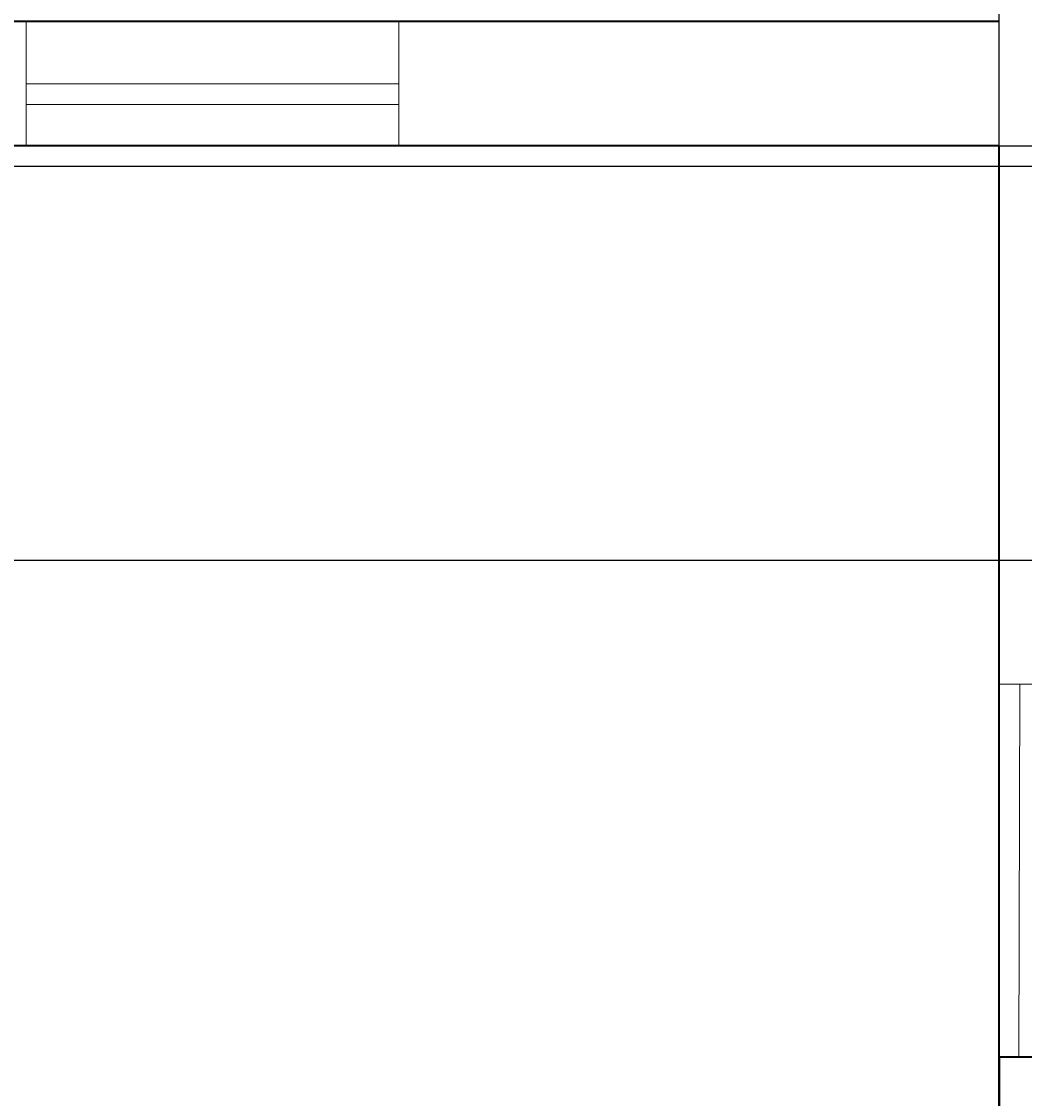
# Model space of a CAD drawing. Units: feet. Extents: x 105 to 1094, y -88 to 588.
# Tile 17 of 59: x 323 to 372, y 250 to 302. Entities that reach past the tile are written whole.
import ezdxf

# ---------------------------------------------------------------- set-up
doc = ezdxf.new("R2010")
doc.units = ezdxf.units.FT
doc.header["$MEASUREMENT"] = 0
for name, color, linetype, lineweight in [('A-ANNO-DIMS', 2, 'Continuous', 18), ('A-GLAZ', 4, 'Continuous', 18), ('A-WALL', 7, 'Continuous', 35)]:
    doc.layers.add(name, color=color, linetype=linetype, lineweight=lineweight)
doc.styles.get("Standard").update_dxf_attribs({"font": 'arial.ttf'})
doc.dimstyles.get("Standard").update_dxf_attribs({"dimtxt": 0.18, "dimasz": 0.18, "dimexe": 0.18, "dimexo": 0.0625, "dimgap": 0.09, "dimtad": 0, "dimtih": 1, "dimtoh": 1, "dimdec": 4, "dimzin": 0, "dimdsep": 46, "dimtxsty": 'Standard', "dimcen": 0.09, "dimadec": 0, "dimazin": 0, "dimtfac": 1, "dimtdec": 4, "dimtofl": 0, "dimtmove": 0, "dimatfit": 3, "dimfxl": 1, "dimtolj": 1, "dimtzin": 0, "dimarcsym": 0})

# ---------------------------------------------------------------- blocks, each defined once
blk = doc.blocks.new('VENT-TRANSVERSE')
for p, q in [((0, 0), (0, 6)), ((18, 0), (18, 6)), ((0, 3), (18, 3)), ((0, 2), (18, 2))]:
    blk.add_line(p, q)
blk = doc.blocks.new('VENT-LONGITUDINAL')
for p, q in [((0, 18), (4, 18)), ((2.039, 0), (2, 18)), ((3.039, 0.002), (3, 18.002))]:
    blk.add_line(p, q)
blk = doc.blocks.new('*D20')
at = {"layer": 'A-ANNO-DIMS', "color": 0, "lineweight": -2, "transparency": 16777216}
for p, q in [((150.688, 276.019), (150.688, -88.149)), ((1048.688, 276.019), (1048.688, -88.149)), ((150.868, -87.969), (599.399, -87.969)), ((1048.508, -87.969), (599.977, -87.969))]:
    blk.add_line(p, q, dxfattribs=at)
at = {"layer": 'A-ANNO-DIMS', "color": 0, "transparency": 16777216}
for points in [[(150.868, -87.939), (150.868, -87.999), (150.688, -87.969)], [(1048.508, -87.939), (1048.508, -87.999), (1048.688, -87.969)]]:
    blk.add_solid(points, dxfattribs=at)
at = {"layer": 'Defpoints', "color": 0, "transparency": 16777216}
for p in [(150.688, 276.081), (1048.688, 276.081), (1048.688, -87.969)]:
    blk.add_point(p, dxfattribs=at)
at = {"layer": 'A-ANNO-DIMS', "color": 0, "transparency": 16777216, "insert": (599.688, -87.969), "char_height": 0.18, "attachment_point": 5}
blk.add_mtext('\\A1;898', dxfattribs=at)
blk = doc.blocks.new('*D21')
at = {"layer": 'A-ANNO-DIMS', "color": 0, "lineweight": -2, "transparency": 16777216}
for p, q in [((849.626, 543.081), (105.458, 543.081)), ((105.638, 542.901), (105.638, 250.263)), ((105.638, -42.739), (105.638, 249.899)), ((849.626, -42.919), (105.458, -42.919))]:
    blk.add_line(p, q, dxfattribs=at)
at = {"layer": 'A-ANNO-DIMS', "color": 0, "transparency": 16777216}
for points in [[(105.608, 542.901), (105.668, 542.901), (105.638, 543.081)], [(105.608, -42.739), (105.668, -42.739), (105.638, -42.919)]]:
    blk.add_solid(points, dxfattribs=at)
at = {"layer": 'Defpoints', "color": 0, "transparency": 16777216}
for p in [(105.638, 543.081), (849.688, 543.081), (849.688, -42.919)]:
    blk.add_point(p, dxfattribs=at)
at = {"layer": 'A-ANNO-DIMS', "color": 0, "transparency": 16777216, "insert": (105.638, 250.081), "char_height": 0.18, "attachment_point": 5}
blk.add_mtext('\\A1;586', dxfattribs=at)
blk = doc.blocks.new('*D33')
at = {"layer": 'A-ANNO-DIMS', "color": 0, "lineweight": -2, "transparency": 16777216}
for p, q in [((646.626, 395.081), (105.458, 395.081)), ((105.638, 394.901), (105.638, 345.263)), ((105.638, 295.261), (105.638, 344.899)), ((646.626, 295.081), (105.458, 295.081))]:
    blk.add_line(p, q, dxfattribs=at)
at = {"layer": 'A-ANNO-DIMS', "color": 0, "transparency": 16777216}
for points in [[(105.608, 394.901), (105.668, 394.901), (105.638, 395.081)], [(105.608, 295.261), (105.668, 295.261), (105.638, 295.081)]]:
    blk.add_solid(points, dxfattribs=at)
at = {"layer": 'Defpoints', "color": 0, "transparency": 16777216}
for p in [(646.688, 395.081), (105.638, 295.081), (646.688, 295.081)]:
    blk.add_point(p, dxfattribs=at)
at = {"layer": 'A-ANNO-DIMS', "color": 0, "transparency": 16777216, "insert": (105.638, 345.081), "char_height": 0.18, "attachment_point": 5}
blk.add_mtext('\\A1;100', dxfattribs=at)
blk = doc.blocks.new('*D39')
at = {"layer": 'A-ANNO-DIMS', "color": 0, "lineweight": -2, "transparency": 16777216}
for p, q in [((294.688, 204.144), (294.688, 588.311)), ((294.868, 588.131), (332.47, 588.131)), ((370.508, 588.131), (332.906, 588.131)), ((370.688, 204.144), (370.688, 588.311))]:
    blk.add_line(p, q, dxfattribs=at)
at = {"layer": 'A-ANNO-DIMS', "color": 0, "transparency": 16777216}
for points in [[(294.868, 588.161), (294.868, 588.101), (294.688, 588.131)], [(370.508, 588.161), (370.508, 588.101), (370.688, 588.131)]]:
    blk.add_solid(points, dxfattribs=at)
at = {"layer": 'Defpoints', "color": 0, "transparency": 16777216}
for p in [(370.688, 588.131), (294.688, 204.081), (370.688, 204.081)]:
    blk.add_point(p, dxfattribs=at)
at = {"layer": 'A-ANNO-DIMS', "color": 0, "transparency": 16777216, "insert": (332.688, 588.131), "char_height": 0.18, "attachment_point": 5}
blk.add_mtext('\\A1;76', dxfattribs=at)
blk = doc.blocks.new('*D54')
at = {"layer": 'A-ANNO-DIMS', "color": 0, "lineweight": -2, "transparency": 16777216}
for p, q in [((294.751, 296.081), (1093.918, 296.081)), ((1093.738, 295.901), (1093.738, 286.263)), ((1093.738, 276.261), (1093.738, 285.899)), ((294.751, 276.081), (1093.918, 276.081))]:
    blk.add_line(p, q, dxfattribs=at)
at = {"layer": 'A-ANNO-DIMS', "color": 0, "transparency": 16777216}
for points in [[(1093.708, 295.901), (1093.768, 295.901), (1093.738, 296.081)], [(1093.708, 276.261), (1093.768, 276.261), (1093.738, 276.081)]]:
    blk.add_solid(points, dxfattribs=at)
at = {"layer": 'Defpoints', "color": 0, "transparency": 16777216}
for p in [(294.688, 296.081), (1093.738, 296.081), (294.688, 276.081)]:
    blk.add_point(p, dxfattribs=at)
at = {"layer": 'A-ANNO-DIMS', "color": 0, "transparency": 16777216, "insert": (1093.738, 286.081), "char_height": 0.18, "attachment_point": 5}
blk.add_mtext('\\A1;20', dxfattribs=at)

msp = doc.modelspace()

# ---------------------------------------------------------------- linework, layer by layer
at = {"layer": 'A-WALL'}
for p, q in [((370.6883, 302.0812), (292.6883, 302.0812)), ((370.6883, 296.0812), (294.6883, 296.0812)), ((370.6883, 248.0812), (370.6883, 296.0812)), ((422.6883, 252.0812), (370.6883, 252.0812)), ((552.6883, 252.0812), (370.6883, 252.0812)), ((370.6883, 252.0812), (370.6883, 204.0812))]:
    msp.add_line(p, q, dxfattribs=at)

# ---------------------------------------------------------------- block references
at = {"layer": 'A-GLAZ'}
msp.add_blockref('VENT-TRANSVERSE', (323.688, 296.081), dxfattribs=at)
at = {"layer": 'A-GLAZ', "extrusion": (0, 0, -1), "zscale": -1}
msp.add_blockref('VENT-LONGITUDINAL', (-374.6886, 252.081), dxfattribs=at)

# ---------------------------------------------------------------- dimensions: what is measured, and where the dimension line sits
at = {"layer": 'A-ANNO-DIMS'}
for base, p1, p2, picture, middle in [((370.6883, 588.1312), (294.6883, 204.0812), (370.6883, 204.0812), '*D39', (332.6883, 588.1312)), ((1048.6883, -87.9688), (150.6883, 276.0812), (1048.6883, 276.0812), '*D20', (599.6883, -87.9688))]:
    dim = msp.add_linear_dim(base=base, p1=p1, p2=p2, dimstyle='Standard', override={"dimdec": 0, "dimlfac": 1, "dimrnd": 0, "dimzin": 0, "dimdsep": 46, "dimlunit": 2}, dxfattribs=at)
    dim.commit()
    dim.dimension.update_dxf_attribs({"geometry": picture, "text_midpoint": middle})
for base, p1, p2, picture, middle in [((105.6383, 543.0812), (849.6883, -42.9188), (849.6883, 543.0812), '*D21', (105.6383, 250.0812)), ((105.6383, 295.0812), (646.6883, 395.0812), (646.6883, 295.0812), '*D33', (105.6383, 345.0812)), ((1093.7383, 296.0812), (294.6883, 276.0812), (294.6883, 296.0812), '*D54', (1093.7383, 286.0812))]:
    dim = msp.add_linear_dim(base=base, p1=p1, p2=p2, angle=90, dimstyle='Standard', override={"dimdec": 0, "dimlfac": 1, "dimrnd": 0, "dimzin": 0, "dimdsep": 46, "dimlunit": 2}, dxfattribs=at)
    dim.commit()
    dim.dimension.update_dxf_attribs({"geometry": picture, "text_midpoint": middle})

doc.saveas('drawing.dxf')
